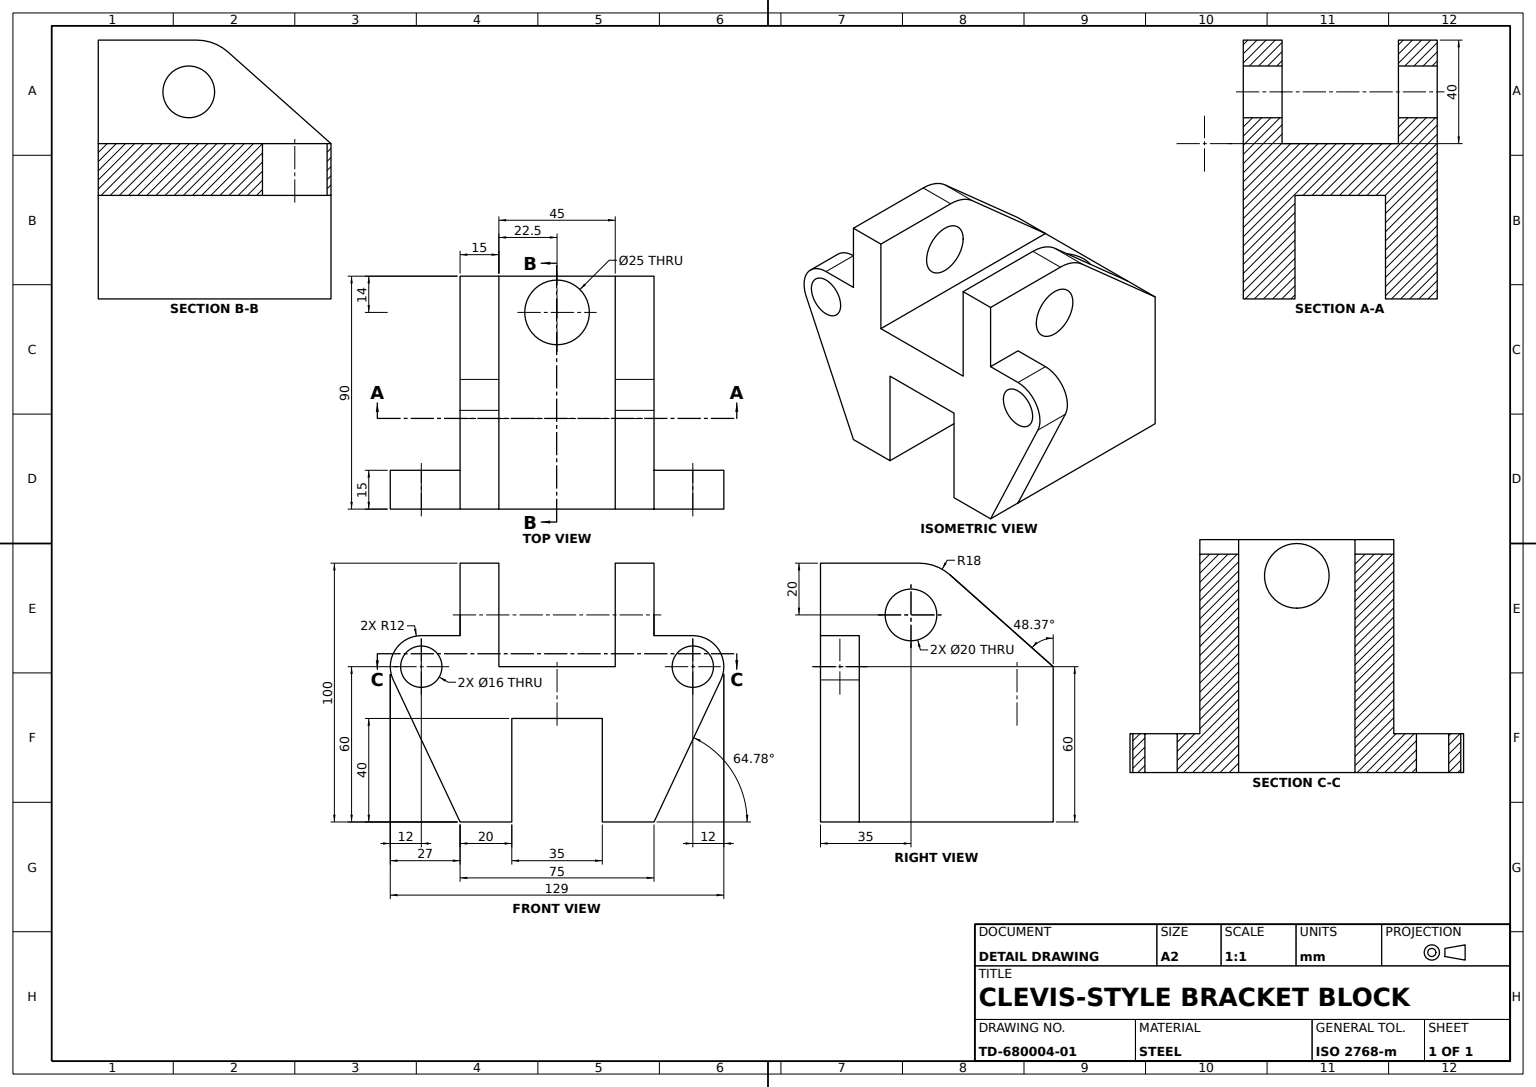
from build123d import *

# Parameters (mm, degrees)
BASE_BLOCK_DEPTH      = 75
BOTTOM_NOTCH_SKETCH_W = 35
BOTTOM_NOTCH_SKETCH_H = 40
BOTTOM_NOTCH_DEPTH    = 155.029218007
TOP_SLOT_SKETCH_W     = 45
TOP_SLOT_SKETCH_H     = 90
TOP_SLOT_DEPTH        = 40
EDGE_FILLET_R18_R     = 18
CROSS_HOLE_SKETCH_R   = 10
CROSS_HOLE_DEPTH      = 155.029218007
PIN_HOLE_SKETCH_R     = 12.5
PIN_HOLE_DEPTH        = 40
SIDE_LUGS_SKETCH_R    = 8
SIDE_LUGS_DEPTH       = 15


with BuildPart() as part:
    # Base Profile Sketch → Base Block (new body)
    with BuildSketch(Plane(origin=(0, 0, 0), x_dir=(0, 0, -1), z_dir=(1, 0, 0))):
        Polygon((0, 0), (90, 0), (90, 60), (45, 100), (0, 100), align=None)
    extrude(amount=-BASE_BLOCK_DEPTH)

    # Bottom Notch Sketch → Bottom Notch (cut, through all)
    with BuildSketch(Plane(origin=(0, 0, -90), x_dir=(-1, 0, 0), z_dir=(0, 0, -1))):
        with Locations((37.5, 20)):
            Rectangle(BOTTOM_NOTCH_SKETCH_W, BOTTOM_NOTCH_SKETCH_H)
    extrude(amount=-BOTTOM_NOTCH_DEPTH, mode=Mode.SUBTRACT)

    # Top Slot Sketch → Top Slot (cut)
    with BuildSketch(Plane(origin=(0, 100, 0), x_dir=(1, 0, 0), z_dir=(0, 1, 0))):
        with Locations((-37.5, 45)):
            Rectangle(TOP_SLOT_SKETCH_W, TOP_SLOT_SKETCH_H)
    extrude(amount=-TOP_SLOT_DEPTH, mode=Mode.SUBTRACT)

    # Edge Fillet R18
    edge_fillet_r18_edges = [part.edges().sort_by_distance(p)[0] for p in [
        (-7.5, 100, -45),
        (-67.5, 100, -45),
    ]]
    fillet(edge_fillet_r18_edges, radius=EDGE_FILLET_R18_R)

    # Cross Hole Sketch → Cross Hole (cut, through all)
    with BuildSketch(Plane(origin=(0, 0, 0), x_dir=(0, 0, -1), z_dir=(1, 0, 0))):
        with Locations((35, 80)):
            Circle(CROSS_HOLE_SKETCH_R)
    extrude(amount=-CROSS_HOLE_DEPTH, mode=Mode.SUBTRACT)

    # Pin Hole Sketch → Pin Hole (cut)
    with BuildSketch(Plane(origin=(0, 60, 0), x_dir=(1, 0, 0), z_dir=(0, 1, 0))):
        with Locations(Location((-37.5, 76, 0), (0, 0, 270))):
            Circle(PIN_HOLE_SKETCH_R)
    extrude(amount=-PIN_HOLE_DEPTH, mode=Mode.SUBTRACT)

    # Side Lugs Sketch → Side Lugs (add)
    # profile 1 of 2: a face of its own
    with BuildSketch(Plane.XY):
        with BuildLine():
            Line((15, 72), (0, 72))
            Line((0, 72), (0, 0))
            Line((0, 0), (25.855763811, 54.886059047))
            ThreePointArc((25.855763811, 54.886059047), (25.133293922, 66.427779888), (15, 72))
        make_face()
        with Locations((15, 60)):
            Circle(SIDE_LUGS_SKETCH_R, mode=Mode.SUBTRACT)
    # profile 2 of 2: a face of its own
    with BuildSketch(Plane.XY):
        with BuildLine():
            Line((-90, 72), (-75, 72))
            Line((-75, 72), (-75, 0))
            Line((-75, 0), (-100.855763811, 54.886059047))
            ThreePointArc((-100.855763811, 54.886059047), (-100.133293922, 66.427779888), (-90, 72))
        make_face()
        with Locations((-90, 60)):
            Circle(SIDE_LUGS_SKETCH_R, mode=Mode.SUBTRACT)
    extrude(amount=-SIDE_LUGS_DEPTH)


solid = part.part
